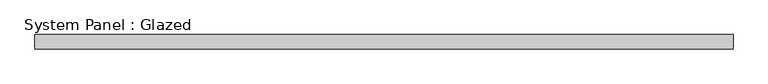
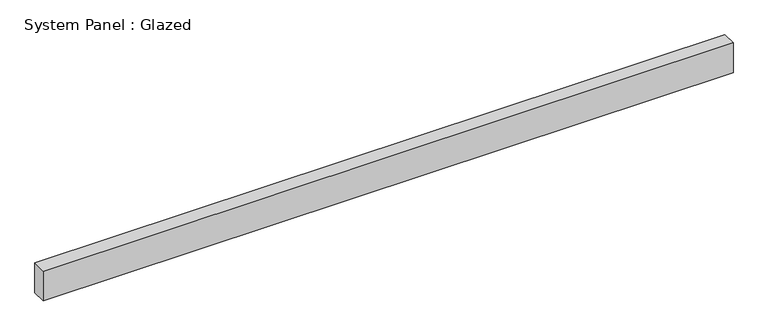
"""IFC4 building model written with IfcOpenShell, lengths in millimetres: plate geometry, System Panel : Glazed."""

from ifc_helpers import new_model, si_unit, origin, origin_with_axes, place, context, project, spatial, polyline, outline, extrude, source, transform, mapped, element, save


def system_panel_glazed_aa2ae1c5(model_context):
    return source(origin(), model_context, "Body", "SweptSolid", [
        extrude(outline(polyline([(622.3, 19.05), (-622.3, 19.05), (-622.3, 44.45), (622.3, 44.45), (622.3, 19.05)])), origin_with_axes(), (0.0, 0.0, 1.0), 57.15),
    ])


if __name__ == "__main__":
    model = new_model("IFC4")
    model_context = context("Model", 3, world=origin())
    ifc_project = project(units=[si_unit("LENGTHUNIT", "METRE", prefix="MILLI")], contexts=[model_context])
    site = spatial("IfcSite", under=ifc_project)
    building = spatial("IfcBuilding", under=site)
    placement = place(None, origin())
    system_panel_glazed_shape = system_panel_glazed_aa2ae1c5(model_context)
    element("IfcPlate", 1, ObjectType="System Panel : Glazed", at=placement, inside=building, context=model_context, shape_type="MappedRepresentation", body=[
        mapped(system_panel_glazed_shape, transform((0.0, 0.0, 0.0), x_axis=(1.0, 0.0, 0.0), y_axis=(0.0, 1.0, 0.0), z_axis=(0.0, 0.0, 1.0))),
    ])
    save(model, "model.ifc")

# Revit data of these elements
# Type "System Panel : Glazed"
#   Construction Type Id = "GSP4R"
#   Analytic Construction = "1/8 in Pilkington single glazing"
#   Visual Light Transmittance = 0.9
#   Solar Heat Gain Coefficient = 0.86
#   Heat Transfer Coefficient (U) = 1.18115 BTU/(h·ft²·°F)
#   Define Thermal Properties by = 1
# Element 1 (IfcPlate, "System Panel : Glazed")
#   Materials on its faces: "Glass"
# Materials
#   "Glass": class "Glass", colour RGB 0 128 192, transparency 0.75, Description = "Soda Lime Glass", Cost = 0
